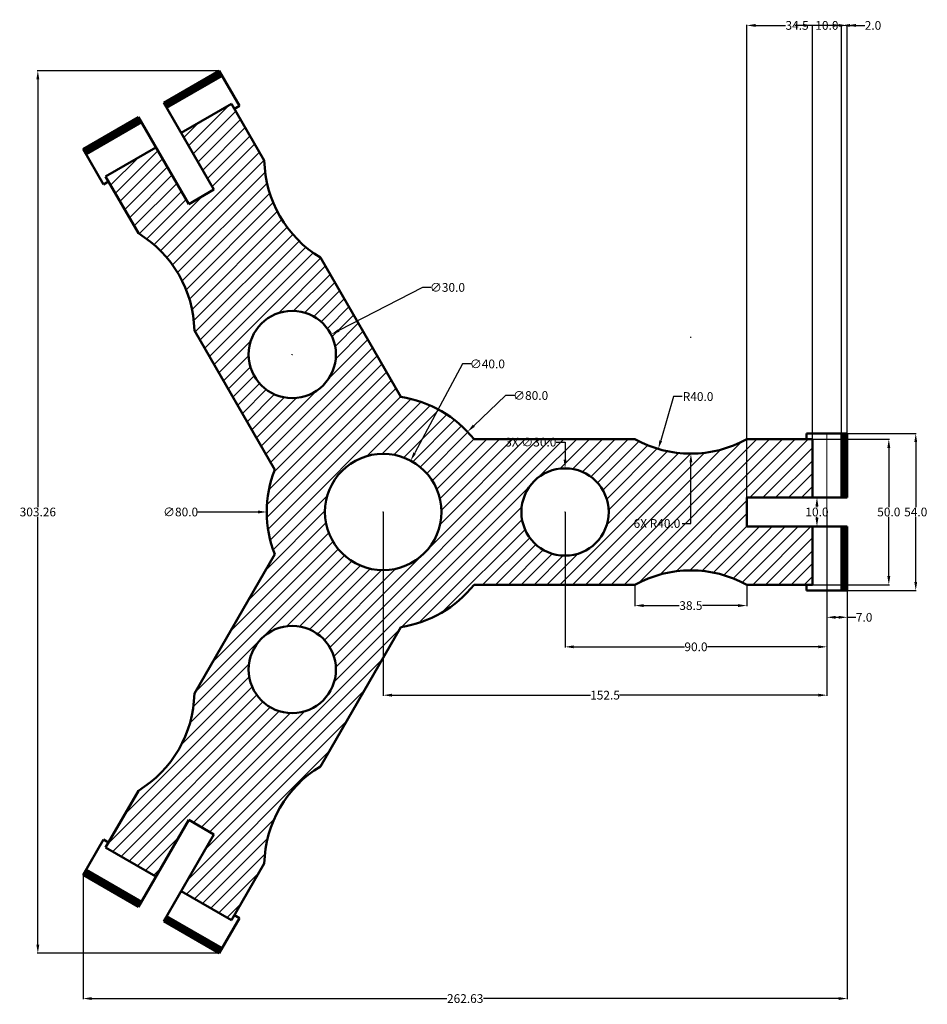
# Model space of a CAD drawing. Units: millimetres. Extents: x 118 to 430, y 14 to 352.
import ezdxf

# ---------------------------------------------------------------- set-up
doc = ezdxf.new("R2010")
doc.units = ezdxf.units.MM
doc.header["$MEASUREMENT"] = 0
for name, color, linetype, lineweight in [('M-CONS', 8, 'Continuous', 13), ('M-DIMS', 3, 'Continuous', 25), ('M-HATC', 8, 'Continuous', 18), ('M-OUTL', 7, 'Continuous', 50)]:
    doc.layers.add(name, color=color, linetype=linetype, lineweight=lineweight)
doc.styles.get("Standard").update_dxf_attribs({"font": 'arial.ttf'})
doc.dimstyles.get("Standard").update_dxf_attribs({"dimtxt": 3, "dimasz": 3, "dimexe": 0.18, "dimexo": 0.0625, "dimgap": 0.09, "dimtad": 0, "dimtih": 1, "dimtoh": 1, "dimdec": 1, "dimzin": 0, "dimdsep": 46, "dimtxsty": 'Standard', "dimcen": 0.09, "dimadec": 0, "dimazin": 0, "dimtfac": 1, "dimtdec": 1, "dimtofl": 0, "dimtmove": 0, "dimatfit": 3, "dimfxl": 1, "dimtolj": 1, "dimtzin": 0, "dimarcsym": 0})

# ---------------------------------------------------------------- blocks, each defined once
blk = doc.blocks.new('*D1')
at = {"layer": 'Defpoints', "color": 0, "transparency": 16777216}
for p in [(243.19, 183.05), (395.69, 183.05), (395.69, 120.11)]:
    blk.add_point(p, dxfattribs=at)
at = {"layer": 'M-DIMS', "color": 0, "lineweight": -2, "transparency": 16777216}
for p, q in [((243.19, 182.98), (243.19, 119.93)), ((395.69, 182.98), (395.69, 119.93)), ((246.19, 120.11), (314.41, 120.11)), ((392.69, 120.11), (324.46, 120.11))]:
    blk.add_line(p, q, dxfattribs=at)
at = {"layer": 'M-DIMS', "color": 0, "transparency": 16777216}
for points in [[(246.19, 120.61), (246.19, 119.61), (243.19, 120.11)], [(392.69, 120.61), (392.69, 119.61), (395.69, 120.11)]]:
    blk.add_solid(points, dxfattribs=at)
at = {"layer": 'M-DIMS', "color": 0, "transparency": 16777216, "insert": (319.44, 120.11), "char_height": 3, "attachment_point": 5}
blk.add_mtext('\\A1;152.5', dxfattribs=at)
blk = doc.blocks.new('*D2')
at = {"layer": 'Defpoints', "color": 0, "transparency": 16777216}
for p in [(305.69, 183.05), (395.69, 183.05), (395.69, 136.72)]:
    blk.add_point(p, dxfattribs=at)
at = {"layer": 'M-DIMS', "color": 0, "lineweight": -2, "transparency": 16777216}
for p, q in [((305.69, 182.98), (305.69, 136.54)), ((395.69, 182.98), (395.69, 136.54)), ((308.69, 136.72), (346.71, 136.72)), ((392.69, 136.72), (354.67, 136.72))]:
    blk.add_line(p, q, dxfattribs=at)
at = {"layer": 'M-DIMS', "color": 0, "transparency": 16777216}
for points in [[(308.69, 137.22), (308.69, 136.22), (305.69, 136.72)], [(392.69, 137.22), (392.69, 136.22), (395.69, 136.72)]]:
    blk.add_solid(points, dxfattribs=at)
at = {"layer": 'M-DIMS', "color": 0, "transparency": 16777216, "insert": (350.69, 136.72), "char_height": 3, "attachment_point": 5}
blk.add_mtext('\\A1;90.0', dxfattribs=at)
blk = doc.blocks.new('*D3')
at = {"layer": 'Defpoints', "color": 0, "transparency": 16777216}
for p in [(395.69, 156.05), (402.69, 156.05), (402.69, 146.87)]:
    blk.add_point(p, dxfattribs=at)
at = {"layer": 'M-DIMS', "color": 0, "lineweight": -2, "transparency": 16777216}
for p, q in [((395.69, 155.98), (395.69, 146.69)), ((402.69, 155.98), (402.69, 146.69)), ((398.69, 146.87), (399.69, 146.87)), ((402.69, 146.87), (405.69, 146.87))]:
    blk.add_line(p, q, dxfattribs=at)
at = {"layer": 'M-DIMS', "color": 0, "transparency": 16777216}
for points in [[(398.69, 147.37), (398.69, 146.37), (395.69, 146.87)], [(399.69, 147.37), (399.69, 146.37), (402.69, 146.87)]]:
    blk.add_solid(points, dxfattribs=at)
at = {"layer": 'M-DIMS', "color": 0, "transparency": 16777216, "insert": (408.49, 146.87), "char_height": 3, "attachment_point": 5}
blk.add_mtext('\\A1;7.0', dxfattribs=at)
blk = doc.blocks.new('*D4')
at = {"layer": 'Defpoints', "color": 0, "transparency": 16777216}
for p in [(390.69, 188.05), (392.27, 188.05), (390.69, 178.05)]:
    blk.add_point(p, dxfattribs=at)
at = {"layer": 'M-DIMS', "color": 0, "lineweight": -2, "transparency": 16777216}
for p, q in [((390.75, 188.05), (392.45, 188.05)), ((392.27, 185.05), (392.27, 184.67)), ((392.27, 181.05), (392.27, 181.43)), ((390.75, 178.05), (392.45, 178.05))]:
    blk.add_line(p, q, dxfattribs=at)
at = {"layer": 'M-DIMS', "color": 0, "transparency": 16777216}
for points in [[(391.77, 185.05), (392.77, 185.05), (392.27, 188.05)], [(391.77, 181.05), (392.77, 181.05), (392.27, 178.05)]]:
    blk.add_solid(points, dxfattribs=at)
at = {"layer": 'M-DIMS', "color": 0, "transparency": 16777216, "insert": (392.27, 183.05), "char_height": 3, "attachment_point": 5}
blk.add_mtext('\\A1;10.0', dxfattribs=at)
blk = doc.blocks.new('*D5')
at = {"layer": 'Defpoints', "color": 0, "transparency": 16777216}
for p in [(390.69, 208.05), (390.69, 158.05), (416.97, 158.05)]:
    blk.add_point(p, dxfattribs=at)
at = {"layer": 'M-DIMS', "color": 0, "lineweight": -2, "transparency": 16777216}
for p, q in [((390.75, 208.05), (417.15, 208.05)), ((416.97, 205.05), (416.97, 184.67)), ((416.97, 161.05), (416.97, 181.43)), ((390.75, 158.05), (417.15, 158.05))]:
    blk.add_line(p, q, dxfattribs=at)
at = {"layer": 'M-DIMS', "color": 0, "transparency": 16777216}
for points in [[(416.47, 205.05), (417.47, 205.05), (416.97, 208.05)], [(416.47, 161.05), (417.47, 161.05), (416.97, 158.05)]]:
    blk.add_solid(points, dxfattribs=at)
at = {"layer": 'M-DIMS', "color": 0, "transparency": 16777216, "insert": (416.97, 183.05), "char_height": 3, "attachment_point": 5}
blk.add_mtext('\\A1;50.0', dxfattribs=at)
blk = doc.blocks.new('*D6')
at = {"layer": 'Defpoints', "color": 0, "transparency": 16777216}
for p in [(402.69, 210.05), (402.69, 156.05), (426.23, 156.05)]:
    blk.add_point(p, dxfattribs=at)
at = {"layer": 'M-DIMS', "color": 0, "lineweight": -2, "transparency": 16777216}
for p, q in [((402.75, 210.05), (426.41, 210.05)), ((426.23, 207.05), (426.23, 184.67)), ((426.23, 159.05), (426.23, 181.43)), ((402.75, 156.05), (426.41, 156.05))]:
    blk.add_line(p, q, dxfattribs=at)
at = {"layer": 'M-DIMS', "color": 0, "transparency": 16777216}
for points in [[(425.73, 207.05), (426.73, 207.05), (426.23, 210.05)], [(425.73, 159.05), (426.73, 159.05), (426.23, 156.05)]]:
    blk.add_solid(points, dxfattribs=at)
at = {"layer": 'M-DIMS', "color": 0, "transparency": 16777216, "insert": (426.23, 183.05), "char_height": 3, "attachment_point": 5}
blk.add_mtext('\\A1;54.0', dxfattribs=at)
blk = doc.blocks.new('*D7')
at = {"layer": 'Defpoints', "color": 0, "transparency": 16777216}
for p in [(225.27, 244.04), (198.6, 230.31)]:
    blk.add_point(p, dxfattribs=at)
at = {"layer": 'M-DIMS', "color": 0, "lineweight": -2, "transparency": 16777216}
for p, q in [((256.68, 260.21), (227.94, 245.41)), ((259.68, 260.21), (256.68, 260.21)), ((211.85, 237.17), (212.03, 237.17)), ((211.94, 237.08), (211.94, 237.26))]:
    blk.add_line(p, q, dxfattribs=at)
at = {"layer": 'M-DIMS', "color": 0, "transparency": 16777216}
blk.add_solid([(227.71, 245.86), (228.17, 244.97), (225.27, 244.04)], dxfattribs=at)
at = {"layer": 'M-DIMS', "color": 0, "transparency": 16777216, "insert": (265.29, 260.21), "char_height": 3, "attachment_point": 5}
blk.add_mtext('\\A1;∅30.0', dxfattribs=at)
blk = doc.blocks.new('*D8')
at = {"layer": 'Defpoints', "color": 0, "transparency": 16777216}
for p in [(252.62, 200.68), (233.75, 165.41)]:
    blk.add_point(p, dxfattribs=at)
at = {"layer": 'M-DIMS', "color": 0, "lineweight": -2, "transparency": 16777216}
for p, q in [((270.4, 233.92), (254.03, 203.33)), ((273.4, 233.92), (270.4, 233.92)), ((243.1, 183.05), (243.28, 183.05)), ((243.19, 182.96), (243.19, 183.14))]:
    blk.add_line(p, q, dxfattribs=at)
at = {"layer": 'M-DIMS', "color": 0, "transparency": 16777216}
blk.add_solid([(253.59, 203.56), (254.48, 203.09), (252.62, 200.68)], dxfattribs=at)
at = {"layer": 'M-DIMS', "color": 0, "transparency": 16777216, "insert": (279.01, 233.92), "char_height": 3, "attachment_point": 5}
blk.add_mtext('\\A1;∅40.0', dxfattribs=at)
blk = doc.blocks.new('*D9')
at = {"layer": 'Defpoints', "color": 0, "transparency": 16777216}
for p in [(272.17, 210.61), (214.2, 155.48)]:
    blk.add_point(p, dxfattribs=at)
at = {"layer": 'M-DIMS', "color": 0, "lineweight": -2, "transparency": 16777216}
for p, q in [((285.27, 223.07), (274.35, 212.68)), ((288.27, 223.07), (285.27, 223.07)), ((243.1, 183.05), (243.28, 183.05)), ((243.19, 182.96), (243.19, 183.14))]:
    blk.add_line(p, q, dxfattribs=at)
at = {"layer": 'M-DIMS', "color": 0, "transparency": 16777216}
blk.add_solid([(274, 213.04), (274.69, 212.32), (272.17, 210.61)], dxfattribs=at)
at = {"layer": 'M-DIMS', "color": 0, "transparency": 16777216, "insert": (293.88, 223.07), "char_height": 3, "attachment_point": 5}
blk.add_mtext('\\A1;∅80.0', dxfattribs=at)
blk = doc.blocks.new('*D10')
at = {"layer": 'Defpoints', "color": 0, "transparency": 16777216}
for p in [(329.69, 158.05), (368.19, 158.05), (368.19, 150.89)]:
    blk.add_point(p, dxfattribs=at)
at = {"layer": 'M-DIMS', "color": 0, "lineweight": -2, "transparency": 16777216}
for p, q in [((329.69, 157.98), (329.69, 150.71)), ((368.19, 157.98), (368.19, 150.71)), ((332.69, 150.89), (344.94, 150.89)), ((365.19, 150.89), (352.93, 150.89))]:
    blk.add_line(p, q, dxfattribs=at)
at = {"layer": 'M-DIMS', "color": 0, "transparency": 16777216}
for points in [[(332.69, 151.39), (332.69, 150.39), (329.69, 150.89)], [(365.19, 151.39), (365.19, 150.39), (368.19, 150.89)]]:
    blk.add_solid(points, dxfattribs=at)
at = {"layer": 'M-DIMS', "color": 0, "transparency": 16777216, "insert": (348.94, 150.89), "char_height": 3, "attachment_point": 5}
blk.add_mtext('\\A1;38.5', dxfattribs=at)
blk = doc.blocks.new('*D11')
at = {"layer": 'Defpoints', "color": 0, "transparency": 16777216}
for p in [(348.94, 243.11), (337.75, 204.71)]:
    blk.add_point(p, dxfattribs=at)
at = {"layer": 'M-DIMS', "color": 0, "lineweight": -2, "transparency": 16777216}
for p, q in [((343, 222.72), (338.59, 207.59)), ((346, 222.72), (343, 222.72))]:
    blk.add_line(p, q, dxfattribs=at)
at = {"layer": 'M-DIMS', "color": 0, "transparency": 16777216}
blk.add_solid([(338.11, 207.73), (339.07, 207.45), (337.75, 204.71)], dxfattribs=at)
at = {"layer": 'M-DIMS', "color": 0, "transparency": 16777216, "insert": (351.41, 222.72), "char_height": 3, "attachment_point": 5}
blk.add_mtext('\\A1;R40.0', dxfattribs=at)
blk = doc.blocks.new('*D12')
at = {"layer": 'Defpoints', "color": 0, "transparency": 16777216}
for p in [(402.69, 156.05), (140.05, 58.42), (402.69, 15.87)]:
    blk.add_point(p, dxfattribs=at)
at = {"layer": 'M-DIMS', "color": 0, "lineweight": -2, "transparency": 16777216}
for p, q in [((402.69, 155.98), (402.69, 15.69)), ((140.05, 58.35), (140.05, 15.69)), ((143.05, 15.87), (265.03, 15.87)), ((399.69, 15.87), (277.71, 15.87))]:
    blk.add_line(p, q, dxfattribs=at)
at = {"layer": 'M-DIMS', "color": 0, "transparency": 16777216}
for points in [[(143.05, 16.37), (143.05, 15.37), (140.05, 15.87)], [(399.69, 16.37), (399.69, 15.37), (402.69, 15.87)]]:
    blk.add_solid(points, dxfattribs=at)
at = {"layer": 'M-DIMS', "color": 0, "transparency": 16777216, "insert": (271.37, 15.87), "char_height": 3, "attachment_point": 5}
blk.add_mtext('\\A1;262.63', dxfattribs=at)
blk = doc.blocks.new('*D13')
at = {"layer": 'Defpoints', "color": 0, "transparency": 16777216}
for p in [(124.5, 334.68), (186.82, 334.68), (186.82, 31.42)]:
    blk.add_point(p, dxfattribs=at)
at = {"layer": 'M-DIMS', "color": 0, "lineweight": -2, "transparency": 16777216}
for p, q in [((186.76, 334.68), (124.32, 334.68)), ((124.5, 331.68), (124.5, 184.67)), ((124.5, 34.42), (124.5, 181.42)), ((186.76, 31.42), (124.32, 31.42))]:
    blk.add_line(p, q, dxfattribs=at)
at = {"layer": 'M-DIMS', "color": 0, "transparency": 16777216}
for points in [[(124, 331.68), (125, 331.68), (124.5, 334.68)], [(124, 34.42), (125, 34.42), (124.5, 31.42)]]:
    blk.add_solid(points, dxfattribs=at)
at = {"layer": 'M-DIMS', "color": 0, "transparency": 16777216, "insert": (124.5, 183.05), "char_height": 3, "attachment_point": 5}
blk.add_mtext('\\A1;303.26', dxfattribs=at)
blk = doc.blocks.new('*D14')
at = {"layer": 'Defpoints', "color": 0, "transparency": 16777216}
for p in [(402.69, 350.23), (368.19, 188.05), (402.69, 188.05)]:
    blk.add_point(p, dxfattribs=at)
at = {"layer": 'M-DIMS', "color": 0, "lineweight": -2, "transparency": 16777216}
for p, q in [((368.19, 188.11), (368.19, 350.41)), ((371.19, 350.23), (381.44, 350.23)), ((399.69, 350.23), (389.43, 350.23)), ((402.69, 188.11), (402.69, 350.41))]:
    blk.add_line(p, q, dxfattribs=at)
at = {"layer": 'M-DIMS', "color": 0, "transparency": 16777216}
for points in [[(371.19, 350.73), (371.19, 349.73), (368.19, 350.23)], [(399.69, 350.73), (399.69, 349.73), (402.69, 350.23)]]:
    blk.add_solid(points, dxfattribs=at)
at = {"layer": 'M-DIMS', "color": 0, "transparency": 16777216, "insert": (385.44, 350.23), "char_height": 3, "attachment_point": 5}
blk.add_mtext('\\A1;34.5', dxfattribs=at)
blk = doc.blocks.new('*D15')
at = {"layer": 'Defpoints', "color": 0, "transparency": 16777216}
for p in [(400.68631, 350.227895), (400.68631, 210.046843), (390.68631, 208.046843)]:
    blk.add_point(p, dxfattribs=at)
at = {"layer": 'M-DIMS', "color": 0, "lineweight": -2, "transparency": 16777216}
for p, q in [((387.68631, 350.227895), (384.68631, 350.227895)), ((390.68631, 208.109343), (390.68631, 350.407895)), ((400.68631, 210.109343), (400.68631, 350.407895)), ((403.68631, 350.227895), (406.68631, 350.227895))]:
    blk.add_line(p, q, dxfattribs=at)
at = {"layer": 'M-DIMS', "color": 0, "transparency": 16777216}
for points in [[(387.68631, 350.727895), (387.68631, 349.727895), (390.68631, 350.227895)], [(403.68631, 350.727895), (403.68631, 349.727895), (400.68631, 350.227895)]]:
    blk.add_solid(points, dxfattribs=at)
at = {"layer": 'M-DIMS', "color": 0, "transparency": 16777216, "insert": (395.68631, 350.227895), "char_height": 3, "attachment_point": 5}
blk.add_mtext('\\A1;10.0', dxfattribs=at)
blk = doc.blocks.new('*D16')
at = {"layer": 'Defpoints', "color": 0, "transparency": 16777216}
for p in [(402.69, 350.23), (400.69, 210.05), (402.69, 210.05)]:
    blk.add_point(p, dxfattribs=at)
at = {"layer": 'M-DIMS', "color": 0, "lineweight": -2, "transparency": 16777216}
for p, q in [((397.69, 350.23), (394.69, 350.23)), ((400.69, 210.11), (400.69, 350.41)), ((402.69, 210.11), (402.69, 350.41)), ((405.69, 350.23), (408.69, 350.23))]:
    blk.add_line(p, q, dxfattribs=at)
at = {"layer": 'M-DIMS', "color": 0, "transparency": 16777216}
for points in [[(397.69, 350.73), (397.69, 349.73), (400.69, 350.23)], [(405.69, 350.73), (405.69, 349.73), (402.69, 350.23)]]:
    blk.add_solid(points, dxfattribs=at)
at = {"layer": 'M-DIMS', "color": 0, "transparency": 16777216, "insert": (411.53, 350.23), "char_height": 3, "attachment_point": 5}
blk.add_mtext('\\A1;2.0', dxfattribs=at)
blk = doc.blocks.new('*D17')
at = {"layer": 'Defpoints', "color": 0, "transparency": 16777216}
for p in [(203.19, 183.05), (283.19, 183.05)]:
    blk.add_point(p, dxfattribs=at)
at = {"layer": 'M-DIMS', "color": 0, "lineweight": -2, "transparency": 16777216}
for p, q in [((179.19, 183.05), (200.19, 183.05)), ((243.1, 183.05), (243.28, 183.05)), ((243.19, 182.96), (243.19, 183.14))]:
    blk.add_line(p, q, dxfattribs=at)
at = {"layer": 'M-DIMS', "color": 0, "transparency": 16777216}
blk.add_solid([(200.19, 183.55), (200.19, 182.55), (203.19, 183.05)], dxfattribs=at)
at = {"layer": 'M-DIMS', "color": 0, "transparency": 16777216, "insert": (173.57, 183.05), "char_height": 3, "attachment_point": 5}
blk.add_mtext('\\A1;∅80.0', dxfattribs=at)
blk = doc.blocks.new('*D18')
at = {"layer": 'Defpoints', "color": 0, "transparency": 16777216}
for p in [(305.69, 198.05), (305.69, 168.05)]:
    blk.add_point(p, dxfattribs=at)
at = {"layer": 'M-DIMS', "color": 0, "lineweight": -2, "transparency": 16777216}
for p, q in [((302.69, 207.05), (305.69, 207.05)), ((305.69, 207.05), (305.69, 201.05)), ((305.6, 183.05), (305.78, 183.05)), ((305.69, 182.96), (305.69, 183.14))]:
    blk.add_line(p, q, dxfattribs=at)
at = {"layer": 'M-DIMS', "color": 0, "transparency": 16777216}
blk.add_solid([(306.19, 201.05), (305.19, 201.05), (305.69, 198.05)], dxfattribs=at)
at = {"layer": 'M-DIMS', "color": 0, "transparency": 16777216, "insert": (293.93, 207.05), "char_height": 3, "attachment_point": 5}
blk.add_mtext('\\A1;3X ∅30.0', dxfattribs=at)
blk = doc.blocks.new('*D19')
at = {"layer": 'Defpoints', "color": 0, "transparency": 16777216}
for p in [(348.94, 243.11), (348.94, 203.11)]:
    blk.add_point(p, dxfattribs=at)
at = {"layer": 'M-DIMS', "color": 0, "lineweight": -2, "transparency": 16777216}
for p, q in [((348.85, 243.11), (349.03, 243.11)), ((348.94, 243.02), (348.94, 243.2)), ((348.94, 179.11), (348.94, 200.11)), ((345.94, 179.11), (348.94, 179.11))]:
    blk.add_line(p, q, dxfattribs=at)
at = {"layer": 'M-DIMS', "color": 0, "transparency": 16777216}
blk.add_solid([(348.44, 200.11), (349.44, 200.11), (348.94, 203.11)], dxfattribs=at)
at = {"layer": 'M-DIMS', "color": 0, "transparency": 16777216, "insert": (337.29, 179.11), "char_height": 3, "attachment_point": 5}
blk.add_mtext('\\A1;6X R40.0', dxfattribs=at)

msp = doc.modelspace()

# ---------------------------------------------------------------- hatches: boundary and pattern name
at = {"layer": 'M-HATC'}
h = msp.add_hatch(dxfattribs=at)
h.set_pattern_fill('ANSI31', color=256, angle=120)
h.set_pattern_definition([(165, (282.39417, 166.10453), (-0.03235238, -0.12074073), [])])
h.paths.add_polyline_path([(140.054, 307.678), (141.054, 305.946), (160.106, 316.946), (159.106, 318.678)])
h.paths.add_polyline_path([(167.766, 323.678), (168.766, 321.946), (187.819, 332.946), (186.819, 334.678)])
h = msp.add_hatch(dxfattribs=at)
h.set_pattern_fill('ANSI31', color=256, scale=25)
h.paths.add_polyline_path([(178.286, 245.458), (205.923, 197.588, 0.1882092), (205.923, 168.505), (178.286, 120.636, -0.2564501), (159.036, 87.294), (147.786, 67.808), (165.106, 57.808), (176.356, 77.294), (185.016, 72.294), (173.766, 52.808), (191.087, 42.808), (202.337, 62.294, -0.2564501), (221.587, 95.636), (249.224, 143.505, 0.1882092), (274.411, 158.047), (329.686, 158.047, -0.2564501), (368.186, 158.047), (390.686, 158.047), (390.686, 178.047), (368.186, 178.047), (368.186, 188.047), (390.686, 188.047), (390.686, 208.047), (368.186, 208.047, -0.2564501), (329.686, 208.047), (274.411, 208.047, 0.1882092), (249.224, 222.588), (221.587, 270.458, -0.2564501), (202.337, 303.8), (191.087, 323.286), (173.766, 313.286), (185.016, 293.8), (176.356, 288.8), (165.106, 308.286), (147.786, 298.286), (159.036, 278.8, -0.2564501)])
h.paths.add_polyline_path([(226.936, 237.173, -1), (196.936, 237.173, -1)], flags=16)
h.paths.add_polyline_path([(263.186, 183.047, -1), (223.186, 183.047, -1)], flags=16)
h.paths.add_polyline_path([(226.936, 128.92, -1), (196.936, 128.92, -1)], flags=16)
h.paths.add_polyline_path([(320.686, 183.047, -1), (290.686, 183.047, -1)], flags=16)
h = msp.add_hatch(dxfattribs=at)
h.set_pattern_fill('ANSI31', color=256)
h.set_pattern_definition([(45, (208.9099, 157.563), (-0.08838835, 0.08838835), [])])
h.paths.add_polyline_path([(402.686, 210.047), (400.686, 210.047), (400.686, 188.047), (402.686, 188.047)])
h.paths.add_polyline_path([(402.686, 178.047), (400.686, 178.047), (400.686, 156.047), (402.686, 156.047)])
h = msp.add_hatch(dxfattribs=at)
h.set_pattern_fill('ANSI31', color=256, angle=-120)
h.set_pattern_definition([(285, (238.25486, 225.473), (0.12074073, 0.03235238), [])])
h.paths.add_polyline_path([(186.819, 31.416), (187.819, 33.148), (168.766, 44.148), (167.766, 42.416)])
h.paths.add_polyline_path([(159.106, 47.416), (160.106, 49.148), (141.054, 60.148), (140.054, 58.416)])

# ---------------------------------------------------------------- linework, layer by layer
at = {"layer": 'M-CONS'}
for p, q in [((395.686, 210.047), (395.686, 188.047)), ((368.186, 183.047), (368.186, 188.047)), ((395.686, 188.047), (395.686, 178.047))]:
    msp.add_line(p, q, dxfattribs=at)
at = {"layer": 'M-OUTL'}
for p, q in [((167.766, 323.678), (186.819, 334.678)), ((168.766, 321.946), (187.819, 332.946)), ((193.819, 322.554), (186.819, 334.678)), ((167.766, 323.678), (185.016, 293.8)), ((191.087, 323.286), (173.766, 313.286)), ((202.337, 303.8), (191.087, 323.286)), ((192.087, 321.554), (193.819, 322.554)), ((140.054, 307.678), (159.106, 318.678)), ((159.106, 318.678), (176.356, 288.8)), ((141.054, 305.946), (160.106, 316.946)), ((165.106, 308.286), (147.786, 298.286)), ((147.054, 295.554), (140.054, 307.678)), ((159.036, 278.8), (147.786, 298.286)), ((147.054, 295.554), (148.786, 296.554)), ((176.356, 288.8), (185.016, 293.8)), ((249.224, 222.588), (221.587, 270.458)), ((205.923, 197.588), (178.286, 245.458)), ((388.686, 210.047), (388.686, 208.047)), ((388.686, 210.047), (402.686, 210.047)), ((400.686, 210.047), (400.686, 188.047)), ((402.686, 210.047), (402.686, 188.047)), ((274.411, 208.047), (329.686, 208.047)), ((368.186, 208.047), (390.686, 208.047)), ((390.686, 188.047), (390.686, 208.047)), ((368.186, 188.047), (368.186, 178.047)), ((402.686, 188.047), (368.186, 188.047)), ((402.686, 178.047), (368.186, 178.047)), ((390.686, 158.047), (390.686, 178.047)), ((400.686, 178.047), (400.686, 156.047)), ((402.686, 178.047), (402.686, 156.047)), ((205.923, 168.505), (178.286, 120.636)), ((274.411, 158.047), (329.686, 158.047)), ((368.186, 158.047), (390.686, 158.047)), ((388.686, 158.047), (388.686, 156.047)), ((388.686, 156.047), (402.686, 156.047)), ((249.224, 143.505), (221.587, 95.636)), ((159.036, 87.294), (147.786, 67.808)), ((159.106, 47.416), (176.356, 77.294)), ((185.016, 72.294), (176.356, 77.294)), ((167.766, 42.416), (185.016, 72.294)), ((147.054, 70.54), (140.054, 58.416)), ((148.786, 69.54), (147.054, 70.54)), ((147.786, 67.808), (165.106, 57.808)), ((202.337, 62.294), (191.087, 42.808)), ((159.106, 47.416), (140.054, 58.416)), ((160.106, 49.148), (141.054, 60.148)), ((173.766, 52.808), (191.087, 42.808)), ((187.819, 33.148), (168.766, 44.148)), ((193.819, 43.54), (192.087, 44.54)), ((186.819, 31.416), (167.766, 42.416)), ((193.819, 43.54), (186.819, 31.416))]:
    msp.add_line(p, q, dxfattribs=at)
for centre, radius in [((211.936, 237.173), 15), ((243.186, 183.047), 20), ((305.686, 183.047), 15), ((211.936, 128.92), 15)]:
    msp.add_circle(centre, radius, dxfattribs=at)
for centre, start, end in [((242.328, 304.661), 181.23293, 238.76707), ((138.295, 244.597), 1.23293, 58.76707), ((243.186, 183.047), 38.68219, 81.31781), ((348.936, 243.11), 241.23293, 298.76707), ((243.186, 183.047), 158.68219, 201.31781), ((348.936, 122.984), 61.23293, 118.76707), ((243.186, 183.047), 278.68219, 321.31781), ((138.295, 121.496), 301.23293, 358.76707), ((242.328, 61.433), 121.23293, 178.76707)]:
    msp.add_arc(centre, 40, start, end, dxfattribs=at)

# ---------------------------------------------------------------- dimensions: what is measured, and where the dimension line sits
at = {"layer": 'M-DIMS'}
for base, p1, p2, override, picture, middle in [((402.686, 350.228), (368.186, 188.047), (402.686, 188.047), {"dimdec": 1, "dimlfac": 1, "dimrnd": 0, "dimzin": 0, "dimdsep": 46, "dimlunit": 2}, '*D14', (385.436, 350.228)), ((400.686, 350.228), (390.686, 208.047), (400.686, 210.047), {"dimdec": 1, "dimlfac": 1, "dimrnd": 0, "dimzin": 0, "dimdsep": 46, "dimlunit": 2}, '*D15', (395.686, 350.228)), ((402.686, 350.228), (400.686, 210.047), (402.686, 210.047), {"dimdec": 1, "dimlfac": 1, "dimrnd": 0, "dimzin": 0, "dimdsep": 46, "dimlunit": 2}, '*D16', (411.528, 350.228)), ((402.686, 15.866), (140.054, 58.416), (402.686, 156.047), {"dimdec": 2, "dimlfac": 1, "dimrnd": 0, "dimzin": 0, "dimdsep": 46, "dimlunit": 2}, '*D12', (271.37, 15.866))]:
    dim = msp.add_linear_dim(base=base, p1=p1, p2=p2, dimstyle='Standard', override=override, dxfattribs=at)
    dim.commit()
    dim.dimension.update_dxf_attribs({"geometry": picture, "text_midpoint": middle})
dim = msp.add_linear_dim(base=(124.504, 334.678), p1=(186.819, 31.416), p2=(186.819, 334.678), angle=90, dimstyle='Standard', override={"dimdec": 2, "dimlfac": 1, "dimrnd": 0, "dimzin": 0, "dimdsep": 46, "dimlunit": 2}, dxfattribs=at)
dim.commit()
dim.dimension.update_dxf_attribs({"geometry": '*D13', "text_midpoint": (124.504, 183.047)})
at = {"layer": 'M-DIMS', "transparency": 33554610}
for p1, p2, picture, middle in [((198.6, 230.307), (225.273, 244.04), '*D7', (265.289, 260.208)), ((233.753, 165.411), (252.619, 200.683), '*D8', (279.013, 233.924)), ((214.201, 155.481), (272.171, 210.613), '*D9', (293.881, 223.068))]:
    dim = msp.add_diameter_dim_2p(p1=p1, p2=p2, dimstyle='Standard', override={"dimclrd": 0, "dimclre": 0, "dimclrt": 0}, dxfattribs=at)
    dim.commit()
    dim.dimension.update_dxf_attribs({"geometry": picture, "text_midpoint": middle, "dimtype": 163})
at = {"layer": 'M-DIMS'}
dim = msp.add_radius_dim(center=(348.936, 243.11), mpoint=(348.936, 203.11), text='6X <>', dimstyle='Standard', override={"dimdec": 1, "dimlfac": 1, "dimrnd": 0, "dimzin": 0, "dimdsep": 46, "dimlunit": 2}, dxfattribs=at)
dim.commit()
dim.dimension.update_dxf_attribs({"geometry": '*D19', "text_midpoint": (337.288, 179.11), "dimtype": 164})
at = {"layer": 'M-DIMS', "transparency": 33554610}
dim = msp.add_radius_dim(center=(348.936, 243.11), mpoint=(337.747, 204.707), dimstyle='Standard', override={"dimclrd": 0, "dimclre": 0, "dimclrt": 0}, dxfattribs=at)
dim.commit()
dim.dimension.update_dxf_attribs({"geometry": '*D11', "text_midpoint": (351.412, 222.719), "dimtype": 164})
at = {"layer": 'M-DIMS'}
dim = msp.add_diameter_dim_2p(p1=(305.687, 168.047), p2=(305.686, 198.047), text='3X <>', dimstyle='Standard', override={"dimdec": 1, "dimlfac": 1, "dimrnd": 0, "dimzin": 0, "dimdsep": 46, "dimlunit": 2}, dxfattribs=at)
dim.commit()
dim.dimension.update_dxf_attribs({"geometry": '*D18', "text_midpoint": (293.93, 207.047), "dimtype": 163})
at = {"layer": 'M-DIMS', "transparency": 33554610}
for base, p1, p2, picture, middle in [((426.227, 156.047), (402.686, 210.047), (402.686, 156.047), '*D6', (426.227, 183.047)), ((416.975, 158.047), (390.686, 208.047), (390.686, 158.047), '*D5', (416.975, 183.047)), ((392.271, 188.047), (390.686, 178.047), (390.686, 188.047), '*D4', (392.271, 183.047))]:
    dim = msp.add_linear_dim(base=base, p1=p1, p2=p2, angle=90, dimstyle='Standard', override={"dimclrd": 0, "dimclre": 0, "dimclrt": 0}, dxfattribs=at)
    dim.commit()
    dim.dimension.update_dxf_attribs({"geometry": picture, "text_midpoint": middle})
at = {"layer": 'M-DIMS'}
dim = msp.add_diameter_dim_2p(p1=(283.186, 183.047), p2=(203.186, 183.047), dimstyle='Standard', override={"dimdec": 1, "dimlfac": 1, "dimrnd": 0, "dimzin": 0, "dimdsep": 46, "dimlunit": 2}, dxfattribs=at)
dim.commit()
dim.dimension.update_dxf_attribs({"geometry": '*D17', "text_midpoint": (179.186, 183.047), "dimtype": 163})
at = {"layer": 'M-DIMS', "transparency": 33554610}
for base, p1, p2, picture, middle in [((395.686, 120.114), (243.186, 183.047), (395.686, 183.047), '*D1', (319.436, 120.114)), ((395.686, 136.721), (305.686, 183.047), (395.686, 183.047), '*D2', (350.686, 136.721)), ((368.186, 150.89), (329.686, 158.047), (368.186, 158.047), '*D10', (348.936, 150.89)), ((402.686, 146.868), (395.686, 156.047), (402.686, 156.047), '*D3', (408.49, 146.868))]:
    dim = msp.add_linear_dim(base=base, p1=p1, p2=p2, dimstyle='Standard', override={"dimclrd": 0, "dimclre": 0, "dimclrt": 0}, dxfattribs=at)
    dim.commit()
    dim.dimension.update_dxf_attribs({"geometry": picture, "text_midpoint": middle})

doc.saveas('drawing.dxf')
